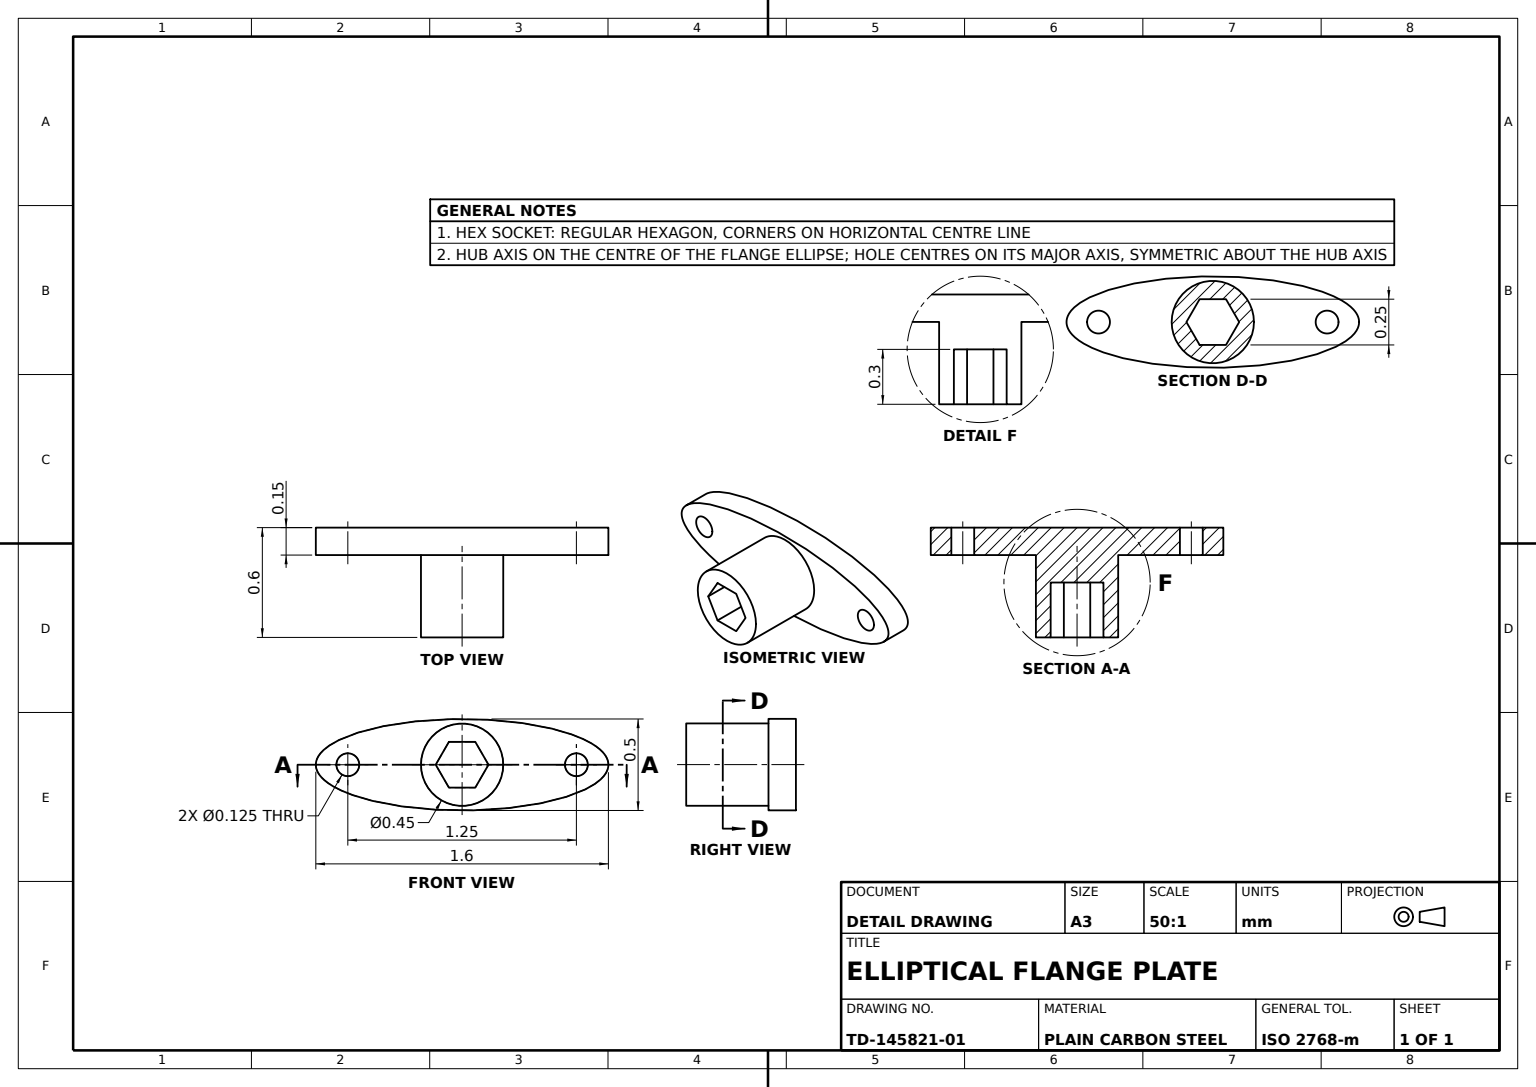
from build123d import *

# Parameters (mm, degrees)
FLANGE_OUTLINE_SKETCH_RX    = 0.8
FLANGE_OUTLINE_SKETCH_RY    = 0.25
OVAL_FLANGE_DEPTH           = 0.15
HUB_AND_HEX_SOCKET_SKETCH_R = 0.225
CYLINDRICAL_HUB_DEPTH       = 0.45
HEX_START                   = 0.45
HEX_SOCKET_DEPTH            = 0.3
MOUNTING_HOLES_SKETCH_R     = 0.0625
MOUNTING_HOLES_2X_DEPTH     = 0.15


with BuildPart() as part:
    # Flange Outline Sketch → Oval Flange (new body)
    with BuildSketch(Plane.XY):
        with Locations((0, 0)):
            Ellipse(FLANGE_OUTLINE_SKETCH_RX, FLANGE_OUTLINE_SKETCH_RY)
    extrude(amount=OVAL_FLANGE_DEPTH)

    # Hub and Hex Socket Sketch → Cylindrical Hub (add)
    with BuildSketch(Plane.XY.offset(0.15)):
        Circle(HUB_AND_HEX_SOCKET_SKETCH_R)
    extrude(amount=CYLINDRICAL_HUB_DEPTH)

    # Sketch2_4 → Hex Socket (cut)
    with BuildSketch(Plane.XY.offset(0.15).offset(HEX_START)):
        Polygon((0.144337567, 0), (0.072168784, 0.125), (-0.072168784, 0.125), (-0.144337567, 0), (-0.072168784, -0.125), (0.072168784, -0.125), align=None)
    extrude(amount=-HEX_SOCKET_DEPTH, mode=Mode.SUBTRACT)

    # Mounting Holes Sketch → Mounting Holes 2x (cut)
    with BuildSketch(Plane(origin=(0, 0, 0), x_dir=(-1, 0, 0), z_dir=(0, 0, -1))):
        with Locations((-0.625, 0)):
            Circle(MOUNTING_HOLES_SKETCH_R)
        with Locations((0.625, 0)):
            Circle(MOUNTING_HOLES_SKETCH_R)
    extrude(amount=-MOUNTING_HOLES_2X_DEPTH, mode=Mode.SUBTRACT)


solid = part.part
